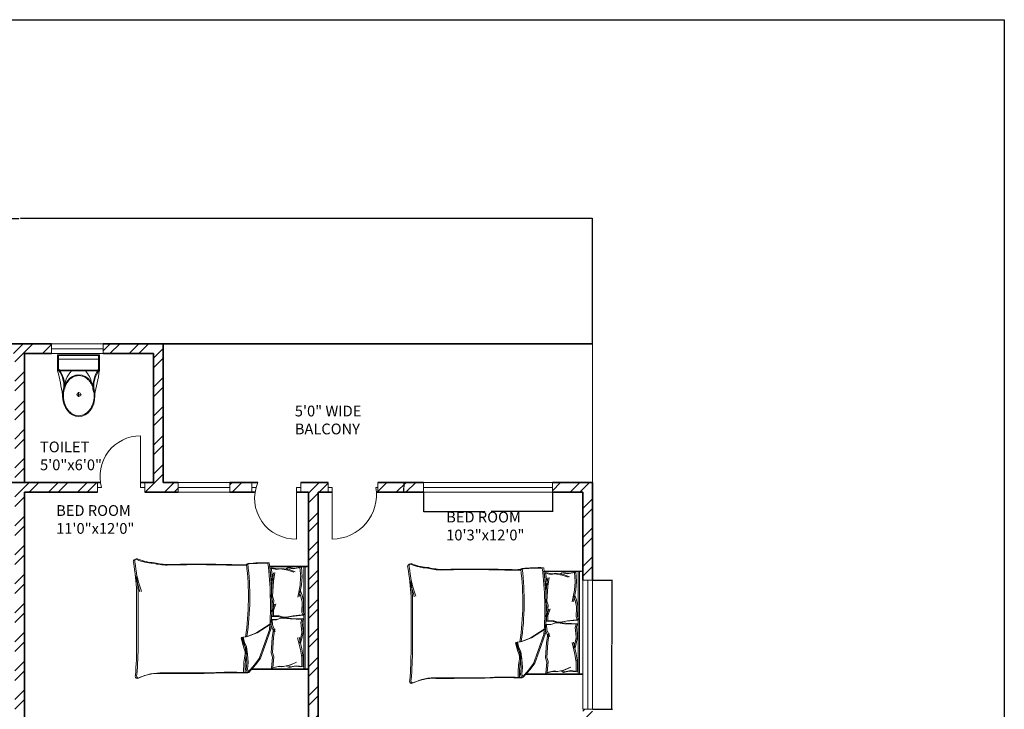
# Model space of a CAD drawing. Units: inches. Extents: x 2168 to 3056, y 1130 to 2629.
# Tile 42 of 42: x 2598 to 3056, y 2308 to 2629. Entities that reach past the tile are written whole.
import ezdxf

# ---------------------------------------------------------------- set-up
doc = ezdxf.new("R2010")
doc.units = ezdxf.units.IN
for name, color, linetype, lineweight in [('A-ANNO-DIMS', 2, 'Continuous', 18), ('A-ANNO-TTLB', 7, 'Continuous', 25), ('A-AREA-IDEN', 7, 'Continuous', 18), ('A-DOOR', 21, 'Continuous', 18), ('A-FLOR-FIXT', 9, 'Continuous', 18), ('A-FLOR-OTLN', 7, 'Continuous', 18), ('A-FURN', 8, 'Continuous', 13), ('A-GLAZ', 201, 'Continuous', 18), ('A-WALL', 7, 'Continuous', 35)]:
    doc.layers.add(name, color=color, linetype=linetype, lineweight=lineweight)
doc.layers.add('A-WALL-PATT', color=143, linetype='Continuous', lineweight=13, true_color=0x7aafdf)
doc.styles.get("Standard").update_dxf_attribs({"font": 'arial.ttf'})
doc.dimstyles.get("Standard").update_dxf_attribs({"dimtxt": 0.18, "dimasz": 0.18, "dimexe": 0.18, "dimexo": 0.0625, "dimgap": 0.09, "dimtad": 0, "dimtih": 1, "dimtoh": 1, "dimdec": 4, "dimzin": 0, "dimdsep": 46, "dimtxsty": 'Standard', "dimcen": 0.09, "dimadec": 0, "dimazin": 0, "dimtfac": 1, "dimtdec": 4, "dimtofl": 0, "dimtmove": 0, "dimatfit": 3, "dimfxl": 1, "dimtolj": 1, "dimtzin": 0, "dimarcsym": 0})

# ---------------------------------------------------------------- blocks, each defined once
blk = doc.blocks.new('A$C31115884')
for p, q in [((283, 498), (223, 498)), ((258, 466), (258, 523)), ((0, 200), (0, 0)), ((520, 200), (0, 200)), ((10, 190), (10, 10)), ((510, 190), (10, 190)), ((510, 10), (510, 190)), ((520, 0), (520, 200)), ((510, 54), (0, 54)), ((10, 10), (510, 10)), ((0, 0), (520, 0))]:
    blk.add_line(p, q)
blk.add_circle((256, 496), 23.6)
for centre, radius, start, end in [((2778, -205), 2807, 165.4549, 171.7133), ((3237, 905), 2807, 188.2867, 194.5451), ((-295, 403), 365, 324.2091, 9.3499), ((-295, 403), 375, 324.2091, 9.3499), ((139, 406), 293, 315.8436, 2.6563), ((806, 403), 375, 179.2036, 215.7909), ((806, 403), 365, 170.6501, 215.7909), ((384, 406), 293, 190.2774, 224.1564)]:
    blk.add_arc(centre, radius, start, end)
blk.add_ellipse((256, 510), major_axis=(0, -261), ratio=0.772727)
blk.add_open_spline([(256, 259), (263, 259), (270, 260), (288, 262), (299, 265), (320, 273), (330, 278), (350, 291), (360, 299), (378, 316), (386, 326), (402, 347), (409, 358), (421, 383), (427, 395), (436, 422), (440, 436), (445, 465), (447, 480), (448, 509), (448, 524), (445, 553), (443, 568), (436, 596), (432, 610), (422, 636), (416, 649), (402, 672), (395, 683), (379, 703), (370, 712), (351, 728), (341, 735), (321, 746), (310, 751), (289, 757), (278, 759), (256, 761), (245, 761), (223, 757), (212, 754), (191, 746), (181, 741), (161, 728), (151, 720), (133, 703), (125, 693), (110, 672), (103, 660), (90, 636), (85, 623), (76, 596), (72, 582), (67, 553), (66, 538), (64, 509), (65, 494), (68, 465), (70, 450), (77, 422), (81, 408), (91, 382), (97, 370), (111, 346), (118, 335), (135, 316), (144, 307), (162, 291), (172, 284), (193, 273), (203, 269), (225, 262), (236, 260), (250, 259), (253, 259), (256, 259)], degree=3, knots=[0, 0, 0, 0, 0.110105, 0.110105, 0.285049, 0.285049, 0.459994, 0.459994, 0.634938, 0.634938, 0.809882, 0.809882, 0.984827, 0.984827, 1.159771, 1.159771, 1.334715, 1.334715, 1.50966, 1.50966, 1.684604, 1.684604, 1.859549, 1.859549, 2.034493, 2.034493, 2.209437, 2.209437, 2.384382, 2.384382, 2.559326, 2.559326, 2.73427, 2.73427, 2.909215, 2.909215, 3.084159, 3.084159, 3.259103, 3.259103, 3.434048, 3.434048, 3.608992, 3.608992, 3.783936, 3.783936, 3.958881, 3.958881, 4.133825, 4.133825, 4.30877, 4.30877, 4.483714, 4.483714, 4.658658, 4.658658, 4.833603, 4.833603, 5.008547, 5.008547, 5.183491, 5.183491, 5.358436, 5.358436, 5.53338, 5.53338, 5.708324, 5.708324, 5.883269, 5.883269, 6.058213, 6.058213, 6.233158, 6.233158, 6.283185, 6.283185, 6.283185, 6.283185])
blk = doc.blocks.new('BED-DOUBLE')
for p, q in [((0, 51.49), (0.64, 51.49)), ((0, 3.48), (0, 51.49)), ((0, 51.27), (26.61, 51.27)), ((0, 51.27), (26.61, 51.27)), ((0.64, 51.49), (27.25, 51.49)), ((0.64, 51.49), (27.25, 51.49)), ((1.53, 3.48), (1.53, 51.27)), ((1.53, 3.48), (1.53, 51.27)), ((2.17, 3.7), (2.17, 51.49)), ((2.17, 3.7), (2.17, 51.49)), ((3.2, 50.34), (3.1, 44.94)), ((3.2, 50.34), (3.1, 44.94)), ((3.2, 50.34), (6.41, 49.96)), ((3.2, 50.34), (6.41, 49.96)), ((6.41, 49.96), (8.98, 50.56)), ((6.41, 49.96), (8.98, 50.56)), ((12.47, 50.34), (8.9, 49.54)), ((12.47, 50.34), (8.9, 49.54)), ((8.98, 50.56), (10.02, 50.04)), ((8.98, 50.56), (10.02, 50.04)), ((14.07, 50.15), (12.47, 50.34)), ((14.07, 50.15), (12.47, 50.34)), ((16.57, 50.7), (13.43, 49.92)), ((16.57, 50.7), (13.43, 49.92)), ((17.21, 50.93), (14.07, 50.15)), ((17.21, 50.93), (14.07, 50.15)), ((16.17, 45.57), (16.57, 50.7)), ((16.17, 45.57), (16.57, 50.7)), ((16.81, 45.8), (17.21, 50.93)), ((16.81, 45.79), (17.21, 50.93)), ((27.75, 52.87), (24.5, 49.16)), ((27.75, 52.87), (24.5, 49.16)), ((28.39, 53.1), (25.14, 49.39)), ((28.39, 53.1), (25.14, 49.39)), ((29.49, 52.95), (27.75, 52.87, 3.87)), ((29.49, 52.95), (27.75, 52.87, 3.87)), ((28.37, 51.33), (27.75, 52.87)), ((28.37, 51.33), (27.75, 52.87)), ((28.06, 48.23), (28.37, 51.33)), ((28.06, 48.23), (28.37, 51.33)), ((30.13, 53.18), (28.39, 53.1, 3.87)), ((30.13, 53.18), (28.39, 53.1, 3.87)), ((29, 51.56), (28.39, 53.1)), ((29, 51.56), (28.39, 53.1)), ((28.7, 48.46), (29, 51.56)), ((28.7, 48.46), (29, 51.56)), ((2.56, 50.11), (2.46, 44.71)), ((2.56, 50.11), (2.46, 44.71)), ((2.56, 50.11), (5.77, 49.73)), ((2.56, 50.11), (5.77, 49.73)), ((3.1, 44.94), (3.18, 45.94)), ((3.1, 44.94), (3.18, 45.94)), ((3.18, 45.94), (3.71, 42.14)), ((3.18, 45.94), (3.71, 42.14)), ((8.26, 49.31), (5.58, 48.13)), ((8.26, 49.31), (5.58, 48.13)), ((5.77, 49.73), (8.34, 50.33)), ((5.77, 49.73), (8.34, 50.33)), ((8.9, 49.54), (6.22, 48.36)), ((8.9, 49.54), (6.22, 48.36)), ((11.83, 50.11), (8.26, 49.31)), ((11.83, 50.11), (8.26, 49.31)), ((8.34, 50.33), (9.38, 49.81)), ((8.34, 50.33), (9.38, 49.81)), ((13.43, 49.92), (11.83, 50.11)), ((13.43, 49.92), (11.83, 50.11)), ((17.37, 43.83), (16.81, 45.8)), ((17.37, 43.83), (16.81, 45.79)), ((22.33, 46.22), (20.32, 40.64)), ((22.33, 46.22), (20.32, 40.64)), ((22.97, 46.45), (20.96, 40.87)), ((22.97, 46.45), (20.96, 40.87)), ((24.5, 49.16), (22.33, 46.22)), ((24.5, 49.16), (22.33, 46.22)), ((25.14, 49.39), (22.97, 46.45)), ((25.14, 49.39), (22.97, 46.45)), ((28.37, 44.36), (28.06, 48.23)), ((28.37, 44.36), (28.06, 48.23)), ((29, 44.59), (28.7, 48.46)), ((29, 44.59), (28.7, 48.46)), ((2.46, 44.71), (2.54, 45.71)), ((2.46, 44.71), (2.54, 45.71)), ((2.54, 45.71), (3.07, 41.91)), ((2.54, 45.71), (3.07, 41.91)), ((3.07, 41.91), (4.42, 36.5)), ((3.07, 41.91), (4.42, 36.49)), ((3.71, 42.14), (5.06, 36.72)), ((3.71, 42.14), (5.06, 36.72)), ((16.73, 43.61), (16.17, 45.57)), ((16.73, 43.61), (16.17, 45.57)), ((16.3, 36.6), (16.73, 43.61)), ((16.3, 36.6), (16.73, 43.61)), ((16.93, 36.82), (17.37, 43.83)), ((16.93, 36.82), (17.37, 43.83)), ((28.83, 40.95), (28.37, 44.36)), ((28.83, 40.95), (28.37, 44.36)), ((29.47, 41.18), (29, 44.59)), ((29.47, 41.18), (29, 44.59)), ((30.4, 39.17), (29.47, 41.18)), ((30.4, 39.17), (29.47, 41.18)), ((3.08, 37.14), (2.54, 34.2)), ((3.08, 37.14), (2.54, 34.2)), ((3.67, 39.2), (3.08, 37.14)), ((3.67, 39.2), (3.08, 37.14)), ((3.72, 37.36), (3.18, 34.43)), ((3.72, 37.36), (3.18, 34.43)), ((4.31, 39.43), (3.72, 37.36)), ((4.31, 39.43), (3.72, 37.36)), ((16.27, 32.79), (16.93, 36.82)), ((16.27, 32.79), (16.93, 36.82)), ((20.32, 40.64), (17.38, 32.31)), ((20.32, 40.64), (17.38, 32.31)), ((20.96, 40.87), (18.02, 32.53)), ((20.96, 40.87), (18.02, 32.53)), ((29.76, 38.94), (28.83, 40.95)), ((29.76, 38.94), (28.83, 40.95)), ((29, 36.38), (31.02, 36.69)), ((29, 36.38), (31.02, 36.69)), ((30.38, 36.46), (29.76, 38.94)), ((30.38, 36.46), (29.76, 38.94)), ((31.02, 36.69), (30.4, 39.17)), ((31.02, 36.69), (30.4, 39.17)), ((79.25, 15.06), (79.25, 39.68)), ((79.25, 15.06), (79.25, 39.68)), ((79.88, 15.29), (79.88, 39.91)), ((79.88, 15.29), (79.88, 39.91)), ((2.54, 34.2), (2.56, 33.88)), ((2.54, 34.2), (2.56, 33.88)), ((2.56, 33.88), (2.98, 29.46)), ((2.56, 33.88), (2.98, 29.46)), ((3.18, 34.43), (3.2, 34.11)), ((3.18, 34.43), (3.2, 34.11)), ((3.2, 34.11), (3.62, 29.68)), ((3.2, 34.11), (3.62, 29.68)), ((16.74, 30.75), (15.45, 33.82)), ((16.74, 30.75), (15.45, 33.82)), ((15.63, 32.56), (16.3, 36.6)), ((15.63, 32.56), (16.3, 36.6)), ((17.38, 30.98), (16.09, 34.05)), ((17.38, 30.98), (16.09, 34.05)), ((17.38, 30.26), (23.88, 34.45)), ((17.38, 30.26), (23.88, 34.45)), ((18.02, 30.49), (24.52, 34.68)), ((18.02, 30.49), (24.52, 34.68)), ((23.88, 34.45), (28.37, 36.15)), ((23.88, 34.45), (28.37, 36.15)), ((24.52, 34.68), (29, 36.38)), ((24.52, 34.68), (29, 36.38)), ((28.37, 36.15), (30.38, 36.46)), ((28.37, 36.15), (30.38, 36.46)), ((2.98, 29.46), (2.49, 27.98)), ((2.98, 29.46), (2.49, 27.98)), ((2.49, 27.98), (7.87, 27.73)), ((2.49, 27.98), (7.87, 27.73)), ((3.62, 29.68), (3.13, 28.21)), ((3.62, 29.68), (3.13, 28.21)), ((3.13, 28.21), (8.51, 27.96)), ((3.13, 28.21), (8.51, 27.96)), ((7.87, 27.73), (11.08, 27.36)), ((7.87, 27.73), (11.08, 27.35)), ((8.51, 27.96), (11.72, 27.58)), ((8.51, 27.96), (11.72, 27.58)), ((11.72, 27.58), (13.02, 27.66)), ((11.72, 27.58), (13.02, 27.66)), ((12.38, 27.44), (14.22, 28.13)), ((12.38, 27.44), (14.22, 28.13)), ((13.02, 27.66), (14.86, 28.36)), ((13.02, 27.66), (14.86, 28.36)), ((14.22, 28.13), (16.89, 28.3)), ((14.22, 28.13), (16.89, 28.3)), ((14.86, 28.36), (17.53, 28.53)), ((14.86, 28.36), (17.53, 28.53)), ((16.89, 28.3), (16.74, 30.75)), ((16.89, 28.3), (16.74, 30.75)), ((17.53, 28.53), (17.38, 30.98)), ((17.53, 28.53), (17.38, 30.98)), ((1.87, 25.98), (7.22, 26.56)), ((1.87, 25.98), (7.22, 26.56)), ((2.45, 24.54), (1.87, 25.98)), ((2.45, 24.54), (1.87, 25.98)), ((2.3, 20.09), (2.45, 24.54)), ((2.3, 20.09), (2.45, 24.54)), ((2.51, 26.21), (7.86, 26.79)), ((2.51, 26.21), (7.86, 26.79)), ((3.09, 24.77), (2.51, 26.21)), ((3.09, 24.77), (2.51, 26.21)), ((2.94, 20.32), (3.09, 24.77)), ((2.94, 20.32), (3.09, 24.77)), ((7.22, 26.56), (10.4, 27.14)), ((7.22, 26.56), (10.4, 27.14)), ((7.86, 26.79), (11.04, 27.37)), ((7.86, 26.79), (11.04, 27.37)), ((10.4, 27.14), (11.7, 27.14)), ((10.4, 27.14), (11.7, 27.14)), ((11.04, 27.37), (12.34, 27.37)), ((11.04, 27.37), (12.34, 27.37)), ((11.08, 27.36), (12.38, 27.44)), ((11.08, 27.35), (12.38, 27.44)), ((11.7, 27.14), (13.58, 26.56)), ((11.7, 27.14), (13.58, 26.56)), ((12.34, 27.37), (14.22, 26.79)), ((12.34, 27.37), (14.22, 26.79)), ((13.58, 26.56), (16.26, 26.56)), ((13.58, 26.56), (16.26, 26.56)), ((14.22, 26.79), (16.9, 26.79)), ((14.22, 26.79), (16.9, 26.79)), ((16.26, 24.1), (15.17, 20.96)), ((16.26, 24.1), (15.17, 20.96)), ((16.9, 24.33), (15.81, 21.19)), ((16.9, 24.33), (15.81, 21.19)), ((16.17, 19.38), (16.57, 24.52)), ((16.17, 19.38), (16.57, 24.52)), ((16.26, 26.56), (16.26, 24.1)), ((16.26, 26.56), (16.26, 24.1)), ((16.81, 19.61), (17.21, 24.74)), ((16.81, 19.61), (17.21, 24.74)), ((16.9, 26.79), (16.9, 24.33)), ((16.9, 26.79), (16.9, 24.33)), ((2.3, 19.77), (2.3, 20.09)), ((2.3, 19.77), (2.3, 20.09)), ((3.03, 16.88), (2.3, 19.77)), ((3.03, 16.88), (2.3, 19.77)), ((2.94, 20), (2.94, 20.32)), ((2.94, 20), (2.94, 20.32)), ((3.67, 17.11), (2.94, 20)), ((3.67, 17.11), (2.94, 20)), ((16.73, 17.42), (16.17, 19.38)), ((16.73, 17.42), (16.17, 19.38)), ((17.37, 17.65), (16.81, 19.61)), ((17.37, 17.65), (16.81, 19.61)), ((3.75, 14.86), (3.03, 16.88)), ((3.75, 14.85), (3.03, 16.88)), ((3.32, 12.11), (4.33, 17.6)), ((3.32, 12.11), (4.33, 17.6)), ((4.39, 15.08), (3.67, 17.11)), ((4.39, 15.08), (3.67, 17.11)), ((3.96, 12.34), (4.97, 17.83)), ((3.96, 12.34), (4.97, 17.83)), ((16.3, 10.41), (16.73, 17.42)), ((16.3, 10.41), (16.73, 17.42)), ((16.93, 10.64), (17.37, 17.65)), ((16.93, 10.64), (17.37, 17.65)), ((3.03, 8.29), (3.32, 12.11)), ((3.03, 8.28), (3.32, 12.11)), ((3.67, 8.51), (3.96, 12.34)), ((3.67, 8.51), (3.96, 12.34)), ((15.63, 6.38), (16.3, 10.41)), ((15.63, 6.38), (16.3, 10.41)), ((16.27, 6.61), (16.93, 10.64)), ((16.27, 6.61), (16.93, 10.64)), ((16.3, 10.41), (16.62, 9.28)), ((16.3, 10.41), (16.62, 9.28)), ((16.62, 9.28), (17.34, 4.18)), ((16.62, 9.28), (17.34, 4.18)), ((16.93, 10.64), (17.26, 9.51)), ((16.93, 10.64), (17.26, 9.51)), ((17.26, 9.51), (17.98, 4.41)), ((17.26, 9.51), (17.98, 4.41)), ((3.01, 8.18), (3.03, 8.29)), ((3.01, 8.18), (3.03, 8.28)), ((3.34, 3.9), (3.01, 8.18)), ((3.34, 3.9), (3.01, 8.18)), ((3.65, 8.41), (3.67, 8.51)), ((3.65, 8.41), (3.67, 8.51)), ((3.98, 4.13), (3.65, 8.41)), ((3.98, 4.13), (3.65, 8.41)), ((3.96, 4.12), (7.14, 4.7)), ((3.96, 4.12), (7.14, 4.7)), ((8.96, 5.05), (6.21, 6.06)), ((8.96, 5.05), (6.21, 6.06)), ((9.59, 5.28), (6.85, 6.29)), ((9.59, 5.28), (6.85, 6.29)), ((7.14, 4.7), (9.74, 4.27)), ((7.14, 4.7), (9.74, 4.27)), ((12.57, 4.47), (8.96, 5.05)), ((12.57, 4.47), (8.96, 5.05)), ((9.1, 4.04), (10.11, 4.62)), ((9.1, 4.04), (10.11, 4.62)), ((13.21, 4.7), (9.59, 5.28)), ((13.21, 4.7), (9.59, 5.28)), ((9.74, 4.27), (10.75, 4.85)), ((9.74, 4.27), (10.75, 4.85)), ((14.16, 4.76), (12.57, 4.47)), ((14.16, 4.76), (12.57, 4.47)), ((14.8, 4.99), (13.21, 4.7)), ((14.8, 4.99), (13.21, 4.7)), ((17.34, 4.18), (14.16, 4.76)), ((17.34, 4.18), (14.16, 4.76)), ((17.98, 4.41), (14.8, 4.99)), ((17.98, 4.41), (14.8, 4.99)), ((18.11, 3.48), (0, 3.48)), ((18.11, 3.48), (0, 3.48)), ((18.75, 3.7), (0.64, 3.7)), ((18.75, 3.7), (0.64, 3.7)), ((3.32, 3.89), (6.5, 4.47)), ((3.32, 3.89), (6.5, 4.47)), ((6.5, 4.47), (9.1, 4.04)), ((6.5, 4.47), (9.1, 4.04))]:
    blk.add_line(p, q)
for centre, radius, start, end in [((68.67, 76.16), 23.07, 267.4714, 296.4681), ((68.67, 76.16), 23.07, 267.4714, 296.4681), ((69.31, 76.39), 23.07, 267.4714, 296.4681), ((69.31, 76.39), 23.07, 267.4714, 296.4681), ((78.87, 54.41), 1.1, 332.6588, 86.02), ((78.87, 54.41), 1.1, 332.6588, 86.02), ((79.51, 54.64), 1.1, 332.6588, 86.02), ((79.51, 54.64), 1.1, 332.6588, 86.02), ((-6.66, 51.33), 36.18, 349.8763, 2.5657), ((-6.66, 51.33), 36.18, 349.8763, 2.5657), ((36.32, 182.27), 129.5, 266.9791, 273.8365), ((36.32, 182.27), 129.5, 266.9791, 273.8365), ((-6.02, 51.56), 36.18, 349.8763, 2.5657), ((-6.02, 51.56), 36.18, 349.8763, 2.5657), ((36.95, 182.49), 129.5, 266.9791, 273.8365), ((36.95, 182.49), 129.5, 266.9791, 273.8365), ((67.82, -4508.74), 4561.86, 90.00217, 90.28689), ((67.82, -4508.74), 4561.86, 90.00217, 90.28689), ((68.46, -4508.51), 4561.86, 90.00217, 90.28689), ((68.46, -4508.52), 4561.86, 90.00217, 90.28689), ((212.28, 41.15), 133.04, 174.4998, 180.6351), ((212.28, 41.15), 133.04, 174.4998, 180.6351), ((212.92, 41.38), 133.04, 174.4998, 180.6351), ((212.92, 41.38), 133.04, 174.4998, 180.6351), ((35.07, 43.74), 6.22, 168.6608, 203.7384), ((35.07, 43.74), 6.22, 168.6608, 203.7384), ((1.48, 31.15), 29.65, 10.6617, 19.8806), ((1.48, 31.15), 29.65, 10.6617, 19.8806), ((35.71, 43.97), 6.22, 168.6608, 203.7384), ((35.71, 43.97), 6.22, 168.6608, 203.7384), ((2.12, 31.38), 29.65, 10.6617, 19.8806), ((2.12, 31.38), 29.65, 10.6617, 19.8806), ((30.44, 36.64), 0.185, 250.2464, 1.1377), ((30.44, 36.64), 0.185, 250.2464, 1.1377), ((31.08, 36.86), 0.185, 250.2464, 1.1377), ((31.08, 36.86), 0.185, 250.2464, 1.1377), ((182.05, 21.36), 164.97, 176.0865, 186.7821), ((182.05, 21.36), 164.97, 176.0865, 186.7821), ((182.69, 21.59), 164.97, 176.0865, 186.7821), ((182.69, 21.59), 164.97, 176.0865, 186.7821), ((156.32, 17.76), 129.02, 171.7845, 186.9006), ((156.32, 17.76), 129.02, 171.7845, 186.9006), ((156.96, 17.98), 129.02, 171.7845, 186.9006), ((156.96, 17.98), 129.02, 171.7845, 186.9006), ((-23.71, -17.22), 106.46, 13.3832, 17.7053), ((-23.71, -17.22), 106.46, 13.3832, 17.7053), ((-23.07, -16.99), 106.46, 13.3832, 17.7053), ((-23.07, -16.99), 106.46, 13.3832, 17.7053), ((200.84, 21.43), 121.76, 182.9958, 189.4091), ((200.84, 21.43), 121.76, 182.9958, 189.4091), ((201.48, 21.66), 121.76, 182.9958, 189.4091), ((201.48, 21.66), 121.76, 182.9958, 189.4091), ((20.1, 85.16), 83.31, 268.7218, 275.604), ((20.1, 85.16), 83.31, 268.7218, 275.604), ((20.74, 85.39), 83.31, 268.7218, 275.604), ((20.74, 85.39), 83.31, 268.7218, 275.604), ((31.17, -167.31), 170.11, 88.4762, 91.0082), ((31.17, -167.31), 170.11, 88.4762, 91.0082), ((31.81, -167.08), 170.11, 88.4762, 91.0082), ((31.81, -167.08), 170.11, 88.4762, 91.0082), ((50.61, 484.82), 482.31, 268.2277, 271.7185), ((50.61, 484.82), 482.31, 268.2277, 271.7185), ((51.25, 485.05), 482.31, 268.2277, 271.7185), ((51.25, 485.05), 482.31, 268.2277, 271.7185), ((64.52, -26.9), 29.63, 76.0648, 88.9113), ((64.52, -26.9), 29.63, 76.0648, 88.9113), ((65.15, -26.67), 29.63, 76.0648, 88.9113), ((65.15, -26.67), 29.63, 76.0648, 88.9113), ((70.28, -21.66), 23.56, 67.9751, 86.652), ((70.28, -21.66), 23.56, 67.9751, 86.652), ((70.92, -21.43), 23.56, 67.9751, 86.652), ((70.92, -21.43), 23.56, 67.9751, 86.652), ((79.72, 1.09), 1.09, 236.1736, 23.4781), ((79.72, 1.09), 1.09, 236.1736, 23.4781), ((80.36, 1.32), 1.09, 236.1736, 23.4781), ((80.36, 1.32), 1.09, 236.1736, 23.4781)]:
    blk.add_arc(centre, radius, start, end)
blk = doc.blocks.new('WIN-24-OPPOSED-JAMBS')
for p, q in [((0, 4.5), (0, 0)), ((0, 4.5), (24, 4.5)), ((0, 0), (0, 2.25)), ((0, 2.25), (24, 2.25)), ((24, 2.25), (24, 4.5)), ((24, 4.5), (24, 0)), ((0, 0), (24, 0))]:
    blk.add_line(p, q)
blk = doc.blocks.new('WIN-24')
for p, q in [((0, 0), (0, 4.5)), ((0, 4.5), (0, 2.25)), ((0, 4.5), (24, 4.5)), ((0, 2.25), (24, 2.25)), ((24, 2.25), (24, 4.5)), ((24, 4.5), (24, 0)), ((24, 0), (0, 0))]:
    blk.add_line(p, q)
blk = doc.blocks.new('WIN-60-OPPOSED-JAMBS')
for p, q in [((2.25, 60), (0, 60)), ((0, 60), (4.5, 60)), ((0, 60), (0, 0)), ((2.25, 0), (2.25, 60)), ((4.5, 60), (4.5, 0)), ((0, 0), (4.5, 0)), ((4.5, 0), (2.25, 0))]:
    blk.add_line(p, q)
blk = doc.blocks.new('WIN-60')
for p, q in [((4.5, 60), (0, 60)), ((0, 0), (0, 60)), ((2.25, 0), (2.25, 60)), ((2.25, 60), (4.5, 60)), ((4.5, 60), (4.5, 0)), ((0, 0), (4.5, 0)), ((4.5, 0), (2.25, 0))]:
    blk.add_line(p, q)
blk = doc.blocks.new('*D34')
at = {"layer": 'A-ANNO-DIMS', "color": 0, "lineweight": -2, "transparency": 16777216}
for p, q in [((2785.65, 2409.33), (2785.65, 2400.21)), ((2845.65, 2409.33), (2845.65, 2400.21)), ((2785.83, 2400.39), (2814.21, 2400.39)), ((2845.47, 2400.39), (2817.1, 2400.39))]:
    blk.add_line(p, q, dxfattribs=at)
at = {"layer": 'A-ANNO-DIMS', "color": 0, "transparency": 16777216}
for points in [[(2785.83, 2400.42), (2785.83, 2400.36), (2785.65, 2400.39)], [(2845.47, 2400.42), (2845.47, 2400.36), (2845.65, 2400.39)]]:
    blk.add_solid(points, dxfattribs=at)
at = {"layer": 'Defpoints', "color": 0, "transparency": 16777216}
for p in [(2785.65, 2409.39), (2845.65, 2409.39), (2845.65, 2400.39)]:
    blk.add_point(p, dxfattribs=at)
at = {"layer": 'A-ANNO-DIMS', "color": 0, "transparency": 16777216, "insert": (2815.65, 2400.39), "char_height": 0.18, "attachment_point": 5}
blk.add_mtext('\\A1;OPP. WINDOW 60 TYP.', dxfattribs=at)
blk = doc.blocks.new('*D35')
at = {"layer": 'A-ANNO-DIMS', "color": 0, "lineweight": -2, "transparency": 16777216}
for p, q in [((2785.59, 2413.89), (2776.47, 2413.89)), ((2776.65, 2413.71), (2776.65, 2411.82)), ((2776.65, 2409.57), (2776.65, 2411.46)), ((2785.59, 2409.39), (2776.47, 2409.39))]:
    blk.add_line(p, q, dxfattribs=at)
at = {"layer": 'A-ANNO-DIMS', "color": 0, "transparency": 16777216}
for points in [[(2776.62, 2413.71), (2776.68, 2413.71), (2776.65, 2413.89)], [(2776.62, 2409.57), (2776.68, 2409.57), (2776.65, 2409.39)]]:
    blk.add_solid(points, dxfattribs=at)
at = {"layer": 'Defpoints', "color": 0, "transparency": 16777216}
for p in [(2785.65, 2413.89), (2776.65, 2409.39), (2785.65, 2409.39)]:
    blk.add_point(p, dxfattribs=at)
at = {"layer": 'A-ANNO-DIMS', "color": 0, "transparency": 16777216, "insert": (2776.65, 2411.64), "char_height": 0.18, "attachment_point": 5}
blk.add_mtext('\\A1;5 TYP.', dxfattribs=at)
blk = doc.blocks.new('*D38')
at = {"layer": 'A-ANNO-DIMS', "color": 0, "lineweight": -2, "transparency": 16777216}
for p, q in [((2864.36, 2368.43), (2873.48, 2368.43)), ((2873.3, 2368.25), (2873.3, 2338.61)), ((2873.3, 2308.61), (2873.3, 2338.24)), ((2864.36, 2308.43), (2873.48, 2308.43))]:
    blk.add_line(p, q, dxfattribs=at)
at = {"layer": 'A-ANNO-DIMS', "color": 0, "transparency": 16777216}
for points in [[(2873.27, 2368.25), (2873.33, 2368.25), (2873.3, 2368.43)], [(2873.27, 2308.61), (2873.33, 2308.61), (2873.3, 2308.43)]]:
    blk.add_solid(points, dxfattribs=at)
at = {"layer": 'Defpoints', "color": 0, "transparency": 16777216}
for p in [(2864.3, 2368.43), (2873.3, 2368.43), (2864.3, 2308.43)]:
    blk.add_point(p, dxfattribs=at)
at = {"layer": 'A-ANNO-DIMS', "color": 0, "transparency": 16777216, "insert": (2873.3, 2338.43), "char_height": 0.18, "attachment_point": 5}
blk.add_mtext('\\A1;WINDOW 60 TYP.', dxfattribs=at)
blk = doc.blocks.new('*D40')
at = {"layer": 'A-ANNO-DIMS', "color": 0, "lineweight": -2, "transparency": 16777216}
for p, q in [((2331.8, 2478.45), (2331.8, 2536.87)), ((2331.98, 2536.69), (2597.65, 2536.69)), ((2864.12, 2536.69), (2598.44, 2536.69)), ((2864.3, 2478.45), (2864.3, 2536.87))]:
    blk.add_line(p, q, dxfattribs=at)
at = {"layer": 'A-ANNO-DIMS', "color": 0, "transparency": 16777216}
for points in [[(2331.98, 2536.72), (2331.98, 2536.66), (2331.8, 2536.69)], [(2864.12, 2536.72), (2864.12, 2536.66), (2864.3, 2536.69)]]:
    blk.add_solid(points, dxfattribs=at)
at = {"layer": 'Defpoints', "color": 0, "transparency": 16777216}
for p in [(2864.3, 2536.69), (2331.8, 2478.39), (2864.3, 2478.39)]:
    blk.add_point(p, dxfattribs=at)
at = {"layer": 'A-ANNO-DIMS', "color": 0, "transparency": 16777216, "insert": (2598.05, 2536.69), "char_height": 0.18, "attachment_point": 5}
blk.add_mtext('\\A1;532.5', dxfattribs=at)

msp = doc.modelspace()

# ---------------------------------------------------------------- hatches: boundary and pattern name
at = {"layer": 'A-WALL-PATT'}
h = msp.add_hatch(dxfattribs=at)
h.set_pattern_fill('ANSI32', color=256)
h.paths.add_polyline_path([(2463.8, 2409.39), (2467.39, 2409.39), (2467.39, 2413.89), (2454.77, 2413.89), (2454.77, 2411.64), (2454.77, 2409.39), (2459.3, 2409.39), (2459.3, 2265.39), (2455.64, 2265.39), (2455.64, 2260.89), (2467.35, 2260.89), (2467.35, 2263.14), (2467.35, 2265.39), (2463.8, 2265.39)])
h.paths.add_polyline_path([(2431.6, 2413.89), (2409.65, 2413.89), (2409.65, 2409.39), (2431.6, 2409.39), (2431.6, 2411.64)])
h.paths.add_polyline_path([(2349.65, 2413.89), (2331.8, 2413.89), (2331.8, 2362.67), (2336.3, 2362.67), (2336.3, 2409.39), (2349.65, 2409.39), (2349.65, 2411.64)])
h.paths.add_polyline_path([(2634.15, 2411.64), (2634.15, 2413.89), (2562.29, 2413.89), (2562.29, 2409.39), (2595.8, 2409.39), (2595.8, 2280.31), (2595.83, 2280.31), (2595.83, 2265.39), (2499.91, 2265.39), (2499.91, 2260.89), (2550.8, 2260.89), (2550.8, 2117.31), (2555.3, 2117.31), (2555.3, 2168.08), (2571.93, 2168.08), (2571.93, 2176.89), (2559.8, 2176.89), (2559.8, 2256.39), (2640.8, 2256.39), (2640.8, 2176.89), (2626.43, 2176.89), (2626.43, 2168.08), (2645.3, 2168.08), (2645.3, 2116.64), (2649.8, 2116.64), (2649.8, 2260.89), (2691.25, 2260.89), (2691.25, 2263.14), (2691.25, 2265.39), (2670.65, 2265.39), (2670.65, 2265.36), (2600.3, 2265.36), (2600.3, 2280.26), (2600.3, 2409.39), (2634.15, 2409.39)])
h.paths.add_polyline_path([(2600.3, 2473.89), (2612.84, 2473.89), (2612.84, 2478.39), (2572.64, 2478.39), (2572.64, 2473.89), (2595.8, 2473.89), (2595.8, 2413.89), (2600.3, 2413.89)])
h.paths.add_polyline_path([(2535.8, 2473.89), (2548.64, 2473.89), (2548.64, 2478.39), (2531.4, 2478.39), (2531.4, 2413.89), (2521.6, 2413.89), (2521.6, 2409.39), (2539.24, 2409.39), (2539.24, 2411.64), (2539.24, 2413.89), (2535.8, 2413.89)])
h.paths.add_polyline_path([(2664.8, 2478.39), (2636.84, 2478.39), (2636.84, 2473.89), (2660.3, 2473.89), (2660.3, 2413.89), (2656.17, 2413.89), (2656.17, 2409.39), (2671.68, 2409.39), (2671.68, 2411.64), (2671.68, 2413.89), (2664.8, 2413.89)])
h.paths.add_polyline_path([(2705.94, 2413.89), (2695.68, 2413.89), (2695.68, 2409.39), (2705.94, 2409.39)])
h.paths.add_polyline_path([(2741.35, 2413.89), (2728.73, 2413.89), (2728.73, 2411.64), (2728.73, 2409.39), (2732.3, 2409.39), (2732.3, 2265.39), (2725.73, 2265.39), (2725.73, 2260.89), (2740.92, 2260.89), (2740.92, 2263.14), (2740.92, 2265.39), (2736.8, 2265.39), (2736.8, 2409.39), (2741.35, 2409.39)])
h.paths.add_polyline_path([(2785.65, 2413.89), (2764.55, 2413.89), (2764.49, 2409.39), (2785.65, 2409.39), (2785.65, 2411.64)])
h.paths.add_polyline_path([(2864.3, 2413.89), (2845.65, 2413.89), (2845.65, 2409.39), (2859.8, 2409.39), (2859.8, 2368.43), (2864.3, 2368.43)])
h.paths.add_polyline_path([(2864.3, 2308.43), (2862.05, 2308.43), (2859.8, 2308.43), (2859.8, 2265.39), (2774.48, 2265.39), (2774.48, 2263.14), (2774.48, 2260.89), (2781.8, 2260.89), (2781.8, 2226.65), (2786.3, 2226.65), (2786.3, 2260.89), (2859.8, 2260.89), (2859.8, 2241.35), (2864.3, 2241.35)])
h.paths.add_polyline_path([(2864.3, 2217.35), (2862.05, 2217.35), (2859.8, 2217.35), (2859.8, 2200.89), (2786.3, 2200.89), (2786.3, 2205.93), (2784.05, 2205.93), (2781.8, 2205.93), (2781.8, 2150.97), (2786.3, 2150.97), (2786.3, 2161.89), (2859.8, 2161.89), (2859.8, 2144.42), (2864.3, 2144.42)])
h.paths.add_polyline_path([(2859.8, 2196.39), (2859.8, 2166.39), (2786.3, 2166.39), (2786.3, 2196.39)], flags=16)
h.paths.add_polyline_path([(2864.3, 2108.42), (2862.05, 2108.42), (2859.8, 2108.42), (2859.8, 2080.89), (2786.3, 2080.89), (2786.3, 2111.99), (2781.8, 2111.99), (2781.8, 2080.89), (2649.8, 2080.89), (2649.8, 2086.04), (2647.55, 2086.04), (2645.3, 2086.04), (2645.3, 2071.74), (2649.8, 2071.74), (2649.8, 2076.39), (2781.8, 2076.39), (2781.8, 2041.79), (2786.3, 2041.79), (2786.3, 2076.39), (2859.8, 2076.39), (2859.8, 2058.58), (2864.3, 2058.58)])
h.paths.add_polyline_path([(2864.3, 2022.58), (2859.8, 2022.58), (2859.8, 1992.39), (2786.3, 1992.39), (2786.3, 1999.57), (2781.8, 1999.57), (2781.8, 1848.09), (2784.05, 1848.09), (2786.3, 1848.09), (2786.3, 1851.39), (2859.8, 1851.39), (2859.8, 1838.26), (2864.3, 1838.26)], flags=17)
h.paths.add_polyline_path([(2859.8, 1987.89), (2859.8, 1855.89), (2786.3, 1855.89), (2786.3, 1987.89)], flags=16)
h.paths.add_polyline_path([(2823.05, 1987.89), (2841.42, 1921.89), (2823.05, 1855.89)], flags=0)
h.paths.add_polyline_path([(2864.3, 1814.26), (2859.8, 1814.26), (2859.8, 1791.39), (2786.3, 1791.39), (2786.3, 1825.66), (2784.05, 1825.66), (2781.8, 1825.66), (2781.8, 1791.39), (2720.15, 1791.39), (2720.15, 1791.27), (2649.8, 1791.27), (2649.8, 1806.16), (2649.8, 2038.98), (2647.55, 2038.98), (2645.3, 2038.98), (2645.3, 1783.93), (2649.8, 1783.93), (2649.8, 1786.89), (2781.8, 1786.89), (2781.8, 1746.79), (2786.3, 1746.79), (2786.3, 1786.89), (2859.8, 1786.89), (2859.8, 1770.08), (2864.3, 1770.08)])
h.paths.add_polyline_path([(2864.3, 1734.08), (2862.05, 1734.08), (2859.8, 1734.08), (2859.8, 1705.89), (2786.3, 1705.89), (2786.3, 1714.17), (2781.8, 1714.17), (2781.8, 1660.53), (2786.3, 1660.53), (2786.3, 1666.89), (2859.8, 1666.89), (2859.8, 1648.34), (2864.3, 1648.34)])
h.paths.add_polyline_path([(2786.3, 1701.39), (2859.8, 1701.39), (2859.8, 1671.39), (2786.3, 1671.39)], flags=16)
h.paths.add_polyline_path([(2649.8, 1756.58), (2647.55, 1756.58), (2645.3, 1756.58), (2645.3, 1606.89), (2555.3, 1606.89), (2555.3, 1749.51), (2553.05, 1749.51), (2550.8, 1749.51), (2550.8, 1606.89), (2503.01, 1606.89), (2503.01, 1604.64), (2503.01, 1602.39), (2595.8, 1602.39), (2595.85, 1602.39), (2595.85, 1587.5), (2595.8, 1458.39), (2561.5, 1458.39), (2561.5, 1456.14), (2561.5, 1453.89), (2595.8, 1453.89), (2595.8, 1381.89), (2573.44, 1381.89), (2573.44, 1377.39), (2613.01, 1377.39), (2613.01, 1379.64), (2613.01, 1381.89), (2600.3, 1381.89), (2600.3, 1453.89), (2634.33, 1453.89), (2634.33, 1458.39), (2600.3, 1458.39), (2600.3, 1602.39), (2670.65, 1602.39), (2694.09, 1602.39), (2694.09, 1606.89), (2649.8, 1606.89)])
h.paths.add_polyline_path([(2736.8, 1602.39), (2741.56, 1602.39), (2741.56, 1606.89), (2726.2, 1606.89), (2726.2, 1604.64), (2726.2, 1602.39), (2732.3, 1602.39), (2732.3, 1458.39), (2727.9, 1458.39), (2727.9, 1453.89), (2740.82, 1453.89), (2740.82, 1456.14), (2740.82, 1458.39), (2736.8, 1458.39)])
h.paths.add_polyline_path([(2859.8, 1606.89), (2786.3, 1606.89), (2786.3, 1637.33), (2784.05, 1637.33), (2781.8, 1637.33), (2781.8, 1606.89), (2775.61, 1606.89), (2775.61, 1602.39), (2859.8, 1602.39)])
h.paths.add_polyline_path([(2864.3, 1624.34), (2862.05, 1624.34), (2859.8, 1624.34), (2859.8, 1570.39), (2864.3, 1570.39)])
h.paths.add_polyline_path([(2864.3, 1510.39), (2862.05, 1510.39), (2859.8, 1510.39), (2859.8, 1458.39), (2846.73, 1458.39), (2846.73, 1456.14), (2846.73, 1453.89), (2864.3, 1453.89)])
h.paths.add_polyline_path([(2786.73, 1458.39), (2765.44, 1458.39), (2765.44, 1453.89), (2786.73, 1453.89)])
h.paths.add_polyline_path([(2706, 1458.39), (2695.36, 1458.39), (2695.36, 1453.89), (2706, 1453.89), (2706, 1456.14)])
h.paths.add_polyline_path([(2671.36, 1456.14), (2671.36, 1458.39), (2655.99, 1458.39), (2655.99, 1456.14), (2655.99, 1453.89), (2660.3, 1453.89), (2660.3, 1381.89), (2637.01, 1381.89), (2637.01, 1377.39), (2664.8, 1377.39), (2664.8, 1453.89), (2671.36, 1453.89)], flags=17)
h.paths.add_polyline_path([(2539.83, 1458.39), (2520.24, 1458.39), (2520.24, 1453.89), (2531.3, 1453.89), (2531.3, 1377.39), (2546.45, 1377.39), (2546.45, 1379.64), (2546.45, 1381.89), (2535.8, 1381.89), (2535.8, 1453.89), (2539.83, 1453.89)], flags=17)
h.paths.add_polyline_path([(2496.24, 1458.39), (2489.13, 1458.39), (2489.13, 1453.89), (2496.24, 1453.89), (2496.24, 1456.14)])
h.paths.add_polyline_path([(2467.43, 1456.14), (2467.43, 1458.39), (2463.8, 1458.39), (2463.8, 1602.39), (2468.24, 1602.39), (2468.24, 1605.7), (2468.24, 1606.89), (2454.6, 1606.89), (2454.6, 1602.39), (2459.3, 1602.39), (2459.3, 1458.39), (2454.24, 1458.39), (2454.24, 1453.89), (2467.43, 1453.89)])
h.paths.add_polyline_path([(2431.6, 1456.14), (2431.6, 1458.39), (2411.39, 1458.39), (2411.39, 1453.89), (2431.6, 1453.89)])
h.paths.add_polyline_path([(2351.39, 1458.39), (2336.3, 1458.39), (2336.3, 1490.69), (2334.05, 1490.69), (2331.8, 1490.69), (2331.8, 1453.89), (2351.39, 1453.89), (2351.39, 1456.14)])
h.paths.add_polyline_path([(2336.3, 1629.7), (2331.8, 1629.7), (2331.8, 1552.32), (2336.3, 1552.32), (2336.3, 1602.39), (2406.65, 1602.39), (2423.47, 1602.39), (2423.47, 1606.89), (2418.8, 1606.89), (2418.8, 1643.68), (2416.55, 1643.68), (2414.3, 1643.68), (2414.3, 1606.89), (2336.3, 1606.89)])
h.paths.add_polyline_path([(2418.8, 1714.38), (2414.3, 1714.38), (2414.3, 1705.89), (2336.3, 1705.89), (2336.3, 1731.32), (2334.05, 1731.32), (2331.8, 1731.32), (2331.8, 1653.7), (2334.05, 1653.7), (2336.3, 1653.7), (2336.3, 1666.89), (2414.3, 1666.89), (2414.3, 1663.59), (2418.8, 1663.59)])
h.paths.add_polyline_path([(2336.3, 1701.39), (2414.3, 1701.39), (2414.3, 1671.39), (2336.3, 1671.39)], flags=16)
h.paths.add_polyline_path([(2555.3, 2040.06), (2550.8, 2040.06), (2550.8, 1791.39), (2550.56, 1791.2), (2480.2, 1791.2), (2418.8, 1791.39), (2418.8, 1825.45), (2416.55, 1825.45), (2414.3, 1825.45), (2414.3, 1791.39), (2336.3, 1791.39), (2336.3, 1806.41), (2331.8, 1806.41), (2331.8, 1767.32), (2336.3, 1767.32), (2336.3, 1786.89), (2414.3, 1786.89), (2414.3, 1745.46), (2418.8, 1745.46), (2418.8, 1786.89), (2550.8, 1786.89), (2550.8, 1783.01), (2555.3, 1783.01)])
h.paths.add_polyline_path([(2418.8, 1923.39), (2423.21, 1923.39), (2423.21, 1925.64), (2423.21, 1927.89), (2418.8, 1927.89), (2418.8, 2000.05), (2414.3, 2000.05), (2414.3, 1992.39), (2336.3, 1992.39), (2336.3, 1987.89), (2414.3, 1987.89), (2414.3, 1855.89), (2336.3, 1855.89), (2336.3, 1851.39), (2414.3, 1851.39), (2414.3, 1846.76), (2418.8, 1846.76)], flags=17)
h.paths.add_polyline_path([(2336.3, 2019.29), (2334.05, 2019.29), (2331.8, 2019.29), (2331.8, 1830.41), (2336.3, 1830.41)], flags=17)
h.paths.add_polyline_path([(2550.8, 1927.89), (2453.54, 1927.89), (2453.54, 1925.64), (2453.54, 1923.39), (2550.8, 1923.39)], flags=17)
h.paths.add_polyline_path([(2744.99, 1927.89), (2649.8, 1927.89), (2649.8, 1923.39), (2744.99, 1923.39), (2744.99, 1925.64)], flags=17)
h.paths.add_polyline_path([(2555.3, 2086.46), (2553.05, 2086.46), (2550.8, 2086.46), (2550.8, 2080.89), (2418.8, 2080.89), (2336.3, 2080.89), (2336.3, 2115.4), (2334.05, 2115.4), (2331.8, 2115.4), (2331.8, 2055.29), (2336.3, 2055.29), (2336.3, 2076.39), (2550.8, 2076.39), (2550.8, 2071.54), (2555.3, 2071.54)])
h.paths.add_polyline_path([(2418.8, 2121.39), (2414.3, 2121.39), (2414.3, 2080.89), (2418.8, 2080.89)])
h.paths.add_polyline_path([(2418.8, 2076.39), (2414.3, 2076.39), (2414.3, 2035.12), (2418.8, 2035.12)])
h.paths.add_polyline_path([(2422.87, 2263.14), (2422.87, 2265.39), (2406.65, 2265.39), (2406.65, 2265.36), (2336.3, 2265.36), (2336.3, 2280.25), (2336.3, 2302.67), (2334.05, 2302.67), (2331.8, 2302.67), (2331.8, 2246.85), (2336.3, 2246.85), (2336.3, 2260.89), (2414.3, 2260.89), (2414.3, 2224), (2418.8, 2224), (2418.8, 2260.89), (2422.87, 2260.89)])
h.paths.add_polyline_path([(2418.8, 2204.78), (2416.55, 2204.78), (2414.3, 2204.78), (2414.3, 2200.89), (2336.3, 2200.89), (2336.3, 2220.85), (2331.8, 2220.85), (2331.8, 2151.4), (2336.3, 2151.4), (2336.3, 2161.89), (2414.3, 2161.89), (2414.3, 2153.73), (2418.8, 2153.73)])
h.paths.add_polyline_path([(2414.3, 2196.39), (2414.3, 2166.39), (2336.3, 2166.39), (2336.3, 2196.39)], flags=16)
h.paths.add_polyline_path([(2375.3, 2181.39), (2336.3, 2166.39), (2336.3, 2196.39)], flags=0)
h.paths.add_polyline_path([(2809.6, 2172.34), (2838.8, 2172.34), (2838.8, 2191), (2809.6, 2191)], flags=8)
h.paths.add_polyline_path([(2849.75, 1919.59), (2849.75, 1952.67), (2831.09, 1952.67), (2831.09, 1919.59)], flags=8)
h.paths.add_polyline_path([(2808.87, 1901.97), (2808.87, 1937.85), (2790.15, 1937.85), (2790.15, 1901.97)], flags=8)
h.paths.add_polyline_path([(2806.28, 1671.9), (2835.49, 1671.9), (2835.49, 1690.55), (2806.28, 1690.55)], flags=8)
h.paths.add_polyline_path([(2353.19, 1676.55), (2382.39, 1676.55), (2382.39, 1695.21), (2353.19, 1695.21)], flags=8)
h.paths.add_polyline_path([(2360.08, 1832.31), (2389.24, 1832.31), (2389.24, 1850.97), (2360.08, 1850.97)], flags=25)
h.paths.add_polyline_path([(2354.82, 2167.82), (2384.03, 2167.82), (2384.03, 2186.48), (2354.82, 2186.48)], flags=8)

# ---------------------------------------------------------------- linework, layer by layer
at = {"layer": 'A-ANNO-TTLB'}
msp.add_lwpolyline([(2168.16, 2629.19), (3055.63, 2629.19), (3055.63, 1130.19), (2168.16, 1130.19)], close=True, dxfattribs=at)
at = {"layer": 'A-DOOR'}
for p, q in [((2654.17, 2411.64), (2654.17, 2435.64)), ((2634.15, 2413.89), (2634.15, 2409.39)), ((2634.15, 2409.39), (2634.15, 2411.64)), ((2634.15, 2411.64), (2636.15, 2411.64)), ((2656.17, 2411.64), (2654.17, 2411.64)), ((2656.17, 2413.89), (2656.17, 2409.39)), ((2656.17, 2409.39), (2656.17, 2411.64)), ((2705.94, 2409.39), (2705.94, 2413.89)), ((2705.94, 2413.89), (2705.94, 2411.64)), ((2705.94, 2411.64), (2707.94, 2411.64)), ((2728.73, 2411.64), (2726.73, 2411.64)), ((2726.73, 2411.64), (2726.73, 2387.64)), ((2728.73, 2409.39), (2728.73, 2413.89)), ((2728.73, 2413.89), (2728.73, 2411.64)), ((2741.35, 2409.39), (2741.35, 2413.89)), ((2741.35, 2413.89), (2741.35, 2411.64)), ((2741.35, 2411.64), (2743.35, 2411.64)), ((2743.35, 2411.64), (2743.35, 2387.64)), ((2764.52, 2411.64), (2763.55, 2411.64)), ((2764.49, 2409.39), (2764.55, 2413.89)), ((2705.94, 2409.39), (2705.94, 2409.39))]:
    msp.add_line(p, q, dxfattribs=at)
for centre, radius, start, end in [((2654.17, 2416.88), 18.76, 90, 196.21), ((2726.11, 2406.51), 18.88, 156.9853, 271.8905), ((2743.35, 2408.14), 20.5, 270, 9.8387)]:
    msp.add_arc(centre, radius, start, end, dxfattribs=at)
at = {"layer": 'A-FLOR-OTLN'}
msp.add_line((2864.3, 2478.39), (2864.3, 2413.89), dxfattribs=at)
at = {"layer": 'A-WALL'}
for p, q in [((2572.64, 2478.39), (2612.84, 2478.39)), ((2636.84, 2478.39), (2864.3, 2478.39)), ((2664.8, 2413.89), (2664.8, 2478.39)), ((2600.3, 2473.89), (2600.3, 2413.89)), ((2600.3, 2473.89), (2612.84, 2473.89)), ((2600.3, 2473.89), (2612.84, 2473.89)), ((2636.84, 2473.89), (2660.3, 2473.89)), ((2636.84, 2473.89), (2660.3, 2473.89)), ((2660.3, 2473.89), (2660.3, 2413.89)), ((2560.43, 2413.89), (2635.64, 2413.89)), ((2654.17, 2413.89), (2660.3, 2413.89)), ((2664.8, 2413.89), (2671.68, 2413.89)), ((2695.68, 2413.89), (2708.73, 2413.89)), ((2728.73, 2413.89), (2741.35, 2413.89)), ((2764.55, 2413.89), (2785.65, 2413.89)), ((2845.65, 2413.89), (2864.3, 2413.89)), ((2864.3, 2413.89), (2864.3, 2368.43)), ((2600.3, 2409.39), (2634.15, 2409.39)), ((2600.3, 2409.39), (2600.3, 2265.39)), ((2656.17, 2409.39), (2671.68, 2409.39)), ((2695.68, 2409.39), (2707.45, 2409.39)), ((2726.73, 2409.39), (2732.3, 2409.39)), ((2732.3, 2409.39), (2732.3, 2265.39)), ((2736.8, 2409.39), (2736.8, 2265.39)), ((2736.8, 2409.39), (2743.35, 2409.39)), ((2763.81, 2409.39), (2785.65, 2409.39)), ((2845.65, 2409.39), (2859.8, 2409.39)), ((2859.8, 2409.39), (2859.8, 2368.43))]:
    msp.add_line(p, q, dxfattribs=at)

# ---------------------------------------------------------------- block references
at = {"layer": 'A-FLOR-FIXT', "xscale": 0.0372717239612423, "yscale": 0.0372717239612423, "zscale": 0.0372717239612423, "rotation": 180}
msp.add_blockref('A$C31115884', (2635.08, 2473.32), dxfattribs=at)
at = {"layer": 'A-FURN', "rotation": 180}
for p in [(2732.3, 2378.46), (2859.8, 2376.18)]:
    msp.add_blockref('BED-DOUBLE', p, dxfattribs=at)
at = {"layer": 'A-GLAZ'}
for name, p in [('WIN-24', (2612.84, 2473.89)), ('WIN-24-OPPOSED-JAMBS', (2671.68, 2409.39)), ('WIN-60', (2859.8, 2308.43))]:
    msp.add_blockref(name, p, dxfattribs=at)
at = {"layer": 'A-GLAZ', "rotation": 270}
msp.add_blockref('WIN-60-OPPOSED-JAMBS', (2785.65, 2413.89), dxfattribs=at)

# ---------------------------------------------------------------- texts
at = {"layer": 'A-AREA-IDEN', "char_height": 5, "attachment_point": 1}
for s, width, insert in [('5\'0" WIDE\\PBALCONY', 134.4221, (2725.91, 2449.66)), ('TOILET\\P5\'0"x6\'0"', 58.2421, (2607.5, 2432.98)), ('BED ROOM\\P11\'0"x12\'0"', 180.5672, (2615, 2403.39)), ('BED ROOM\\P10\'3"x12\'0"', 127.4192, (2796.26, 2400.34))]:
    msp.add_mtext_dynamic_manual_height_columns(s, width=width, gutter_width=12.5, heights=[0], dxfattribs=dict(at, insert=insert))

# ---------------------------------------------------------------- dimensions: what is measured, and where the dimension line sits
at = {"layer": 'A-ANNO-DIMS'}
dim = msp.add_linear_dim(base=(2864.3, 2536.69), p1=(2331.8, 2478.39), p2=(2864.3, 2478.39), dimstyle='Standard', override={"dimdec": 1, "dimlfac": 1, "dimrnd": 0, "dimzin": 0, "dimdsep": 46, "dimlunit": 2}, dxfattribs=at)
dim.commit()
dim.dimension.update_dxf_attribs({"geometry": '*D40', "text_midpoint": (2598.05, 2536.69)})
for base, p1, p2, angle, text, picture, middle in [((2776.65482348, 2409.38887054), (2785.65482348, 2413.88887054), (2785.65482348, 2409.38887054), 270, '<> TYP.', '*D35', (2776.65482348, 2411.63887054)), ((2873.3, 2368.43), (2864.3, 2308.43), (2864.3, 2368.43), 90, 'WINDOW <> TYP.', '*D38', (2873.3, 2338.43))]:
    dim = msp.add_linear_dim(base=base, p1=p1, p2=p2, angle=angle, text=text, dimstyle='Standard', override={"dimdec": 0, "dimlfac": 1, "dimrnd": 0, "dimzin": 0, "dimdsep": 46, "dimlunit": 2}, dxfattribs=at)
    dim.commit()
    dim.dimension.update_dxf_attribs({"geometry": picture, "text_midpoint": middle})
dim = msp.add_linear_dim(base=(2845.65, 2400.39), p1=(2785.65, 2409.39), p2=(2845.65, 2409.39), text='OPP. WINDOW <> TYP.', dimstyle='Standard', override={"dimdec": 0, "dimlfac": 1, "dimrnd": 0, "dimzin": 0, "dimdsep": 46, "dimlunit": 2}, dxfattribs=at)
dim.commit()
dim.dimension.update_dxf_attribs({"geometry": '*D34', "text_midpoint": (2815.65, 2400.39)})

doc.saveas('drawing.dxf')
